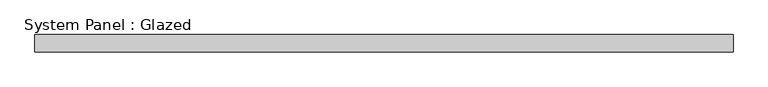
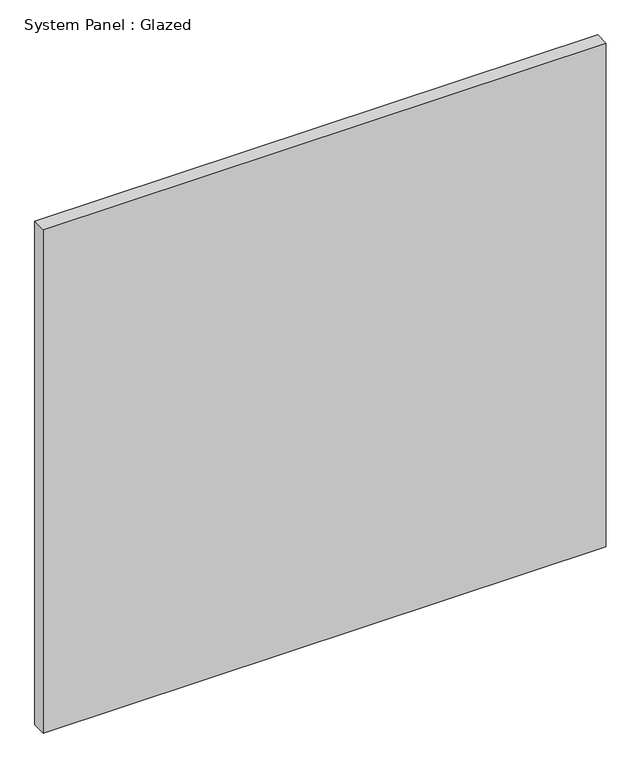
"""IFC4 building model written with IfcOpenShell, lengths in millimetres: plate geometry, System Panel : Glazed."""

from ifc_helpers import new_model, si_unit, origin, origin_with_axes, place, context, project, spatial, polyline, outline, extrude, source, transform, mapped, element, save


def system_panel_glazed_bbd5fb98(model_context):
    return source(origin(), model_context, "Body", "SweptSolid", [
        extrude(outline(polyline([(505.8833333, 19.05), (-505.8833333, 19.05), (-505.8833333, 44.45), (505.8833333, 44.45), (505.8833333, 19.05)])), origin_with_axes(), (0.0, 0.0, 1.0), 956.453622),
    ])


if __name__ == "__main__":
    model = new_model("IFC4")
    model_context = context("Model", 3, world=origin())
    ifc_project = project(units=[si_unit("LENGTHUNIT", "METRE", prefix="MILLI")], contexts=[model_context])
    site = spatial("IfcSite", under=ifc_project)
    building = spatial("IfcBuilding", under=site)
    placement = place(None, origin())
    system_panel_glazed_shape = system_panel_glazed_bbd5fb98(model_context)
    element("IfcPlate", 1, ObjectType="System Panel : Glazed", at=placement, inside=building, context=model_context, shape_type="MappedRepresentation", body=[
        mapped(system_panel_glazed_shape, transform((0.0, 0.0, 0.0), x_axis=(1.0, 0.0, 0.0), y_axis=(0.0, 1.0, 0.0), z_axis=(0.0, 0.0, 1.0))),
    ])
    save(model, "model.ifc")

# Revit data of these elements
# Type "System Panel : Glazed"
#   Construction Type Id = "GSP4R"
#   Analytic Construction = "1/8 in Pilkington single glazing"
#   Visual Light Transmittance = 0.9
#   Solar Heat Gain Coefficient = 0.86
#   Heat Transfer Coefficient (U) = 1.18115 BTU/(h·ft²·°F)
#   Define Thermal Properties by = 1
# Element 1 (IfcPlate, "System Panel : Glazed")
#   Materials on its faces: "Glass"
# Materials
#   "Glass": class "Glass", colour RGB 0 128 192, transparency 0.75, Description = "Soda Lime Glass", Cost = 0
